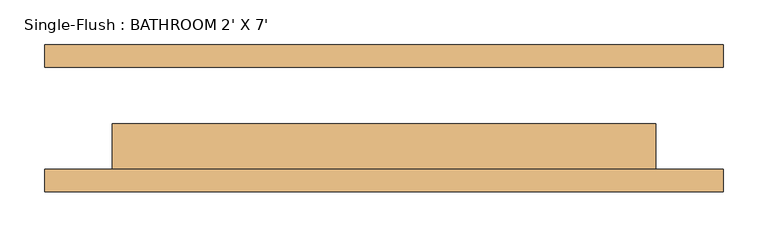
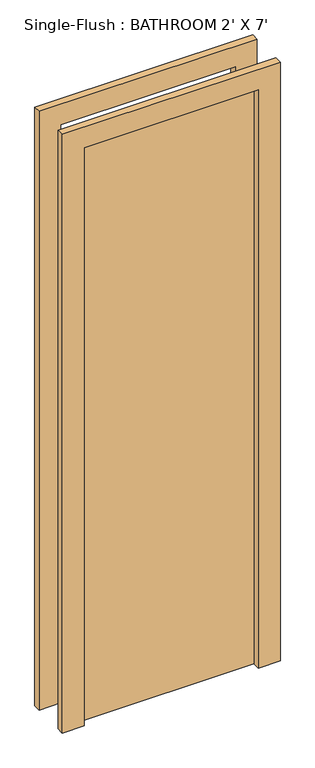
"""IFC4 building model written with IfcOpenShell, lengths in millimetres: door geometry, Single-Flush : BATHROOM 2' X 7'."""

from ifc_helpers import new_model, si_unit, frame, origin, origin_with_axes, place, context, project, spatial, polyline, outline, extrude, source, transform, mapped, element, save


def single_flush_bathroom_2_x_7_0bf9f8da(model_context):
    return source(origin(), model_context, "Body", "SweptSolid", [
        extrude(outline(polyline([(2209.8, -381.0), (0.0, -381.0), (0.0, -304.8), (2133.6, -304.8), (2133.6, 304.8), (0.0, 304.8), (0.0, 381.0), (2209.8, 381.0), (2209.8, -381.0)])), frame((0.0, -82.55, 0.0), z_axis=(0.0, 1.0, 0.0), x_axis=(0.0, 0.0, 1.0)), (0.0, 0.0, 1.0), 25.4),
        extrude(outline(polyline([(2209.8, 381.0), (2209.8, -381.0), (0.0, -381.0), (0.0, -304.8), (2133.6, -304.8), (2133.6, 304.8), (0.0, 304.8), (0.0, 381.0), (2209.8, 381.0)])), frame((0.0, 57.15, 0.0), z_axis=(0.0, 1.0, 0.0), x_axis=(0.0, 0.0, 1.0)), (0.0, 0.0, 1.0), 25.4),
        extrude(outline(polyline([(304.8, -6.35), (304.8, -57.15), (-304.8, -57.15), (-304.8, -6.35), (304.8, -6.35)])), origin_with_axes(), (0.0, 0.0, 1.0), 2133.6),
    ])


if __name__ == "__main__":
    model = new_model("IFC4")
    model_context = context("Model", 3, world=origin())
    ifc_project = project(units=[si_unit("LENGTHUNIT", "METRE", prefix="MILLI")], contexts=[model_context])
    site = spatial("IfcSite", under=ifc_project)
    building = spatial("IfcBuilding", under=site)
    placement = place(None, origin())
    single_flush_bathroom_2_x_7_shape = single_flush_bathroom_2_x_7_0bf9f8da(model_context)
    element("IfcDoor", 1, ObjectType="Single-Flush : BATHROOM 2' X 7'", at=placement, inside=building, context=model_context, shape_type="MappedRepresentation", body=[
        mapped(single_flush_bathroom_2_x_7_shape, transform((0.0, 0.0, 0.0), x_axis=(1.0, 0.0, 0.0), y_axis=(0.0, 1.0, 0.0), z_axis=(0.0, 0.0, 1.0))),
    ])
    save(model, "model.ifc")

# Revit data of these elements
# Type "Single-Flush : BATHROOM 2' X 7'"
#   Type Mark = "8"
#   Construction Type Id = "MDOOR"
#   Assembly Code = "C1020"
#   Analytic Construction = "Metal"
#   Thickness = 0' - 2"
#   Heat Transfer Coefficient (U) = 0.651978 BTU/(h·ft²·°F)
#   Height = 7' - 0"
#   Trim Projection Ext = 0' - 1"
#   Trim Projection Int = 0' - 1"
#   Trim Width = 0' - 3"
#   Width = 2' - 0"
#   Define Thermal Properties by = 1
#   Door Material = Door - Panel
#   Frame Material = Door - Frame
#   Visual Light Transmittance = 0
#   Solar Heat Gain Coefficient = 0
#   Function = (empty or 0)
#   Wall Closure = (empty or 0)
# Element 1 (IfcDoor, "Single-Flush : BATHROOM 2' X 7'")
#   Materials on its faces: "Door - Frame", "Door - Panel"
# Materials
#   "Door - Panel": class "Wood", colour RGB 210 159 95, transparency 0, Cost = 0
#   "Door - Frame": colour RGB 118 70 51, transparency 0, Cost = 0
